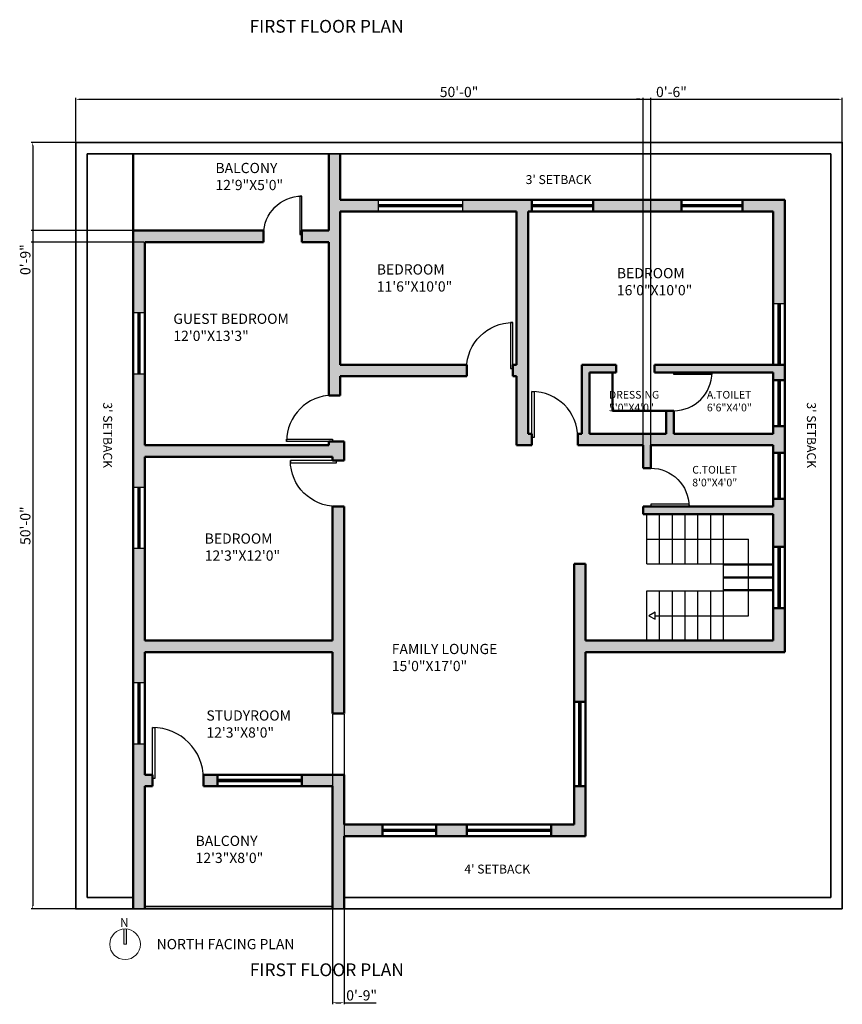
# Model space of a CAD drawing. Units: inches. Extents: x 2442 to 3851, y 589 to 2836.
# Tile 2 of 22: x 3165 to 3809, y 589 to 1359. Entities that reach past the tile are written whole.
import ezdxf

# ---------------------------------------------------------------- set-up
doc = ezdxf.new("R2010")
doc.units = ezdxf.units.IN
for name, color, linetype, lineweight in [('A-ANNO-DIMS', 2, 'Continuous', 18), ('A-ANNO-SYMB', 1, 'Continuous', 18), ('A-ANNO-TEXT', 7, 'Continuous', 18), ('A-AREA-IDEN', 7, 'Continuous', 18), ('A-DOOR', 4, 'Continuous', 25), ('A-FLOR-STRS', 3, 'Continuous', 25), ('A-GLAZ', 1, 'Continuous', 25), ('A-WALL', 7, 'Continuous', 50), ('A-WALL-PATT', 8, 'Continuous', 13), ('C-PROP', 7, 'Continuous', 35)]:
    doc.layers.add(name, color=color, linetype=linetype, lineweight=lineweight)
doc.styles.get("Standard").update_dxf_attribs({"font": 'arial.ttf'})
doc.dimstyles.new('ISO-25', dxfattribs={"dimtxt": 8, "dimasz": 2.5, "dimexe": 1.25, "dimexo": 0.625, "dimtad": 1, "dimlunit": 3, "dimtxsty": 'Standard', "dimcen": 2.5, "dimadec": 0, "dimazin": 0, "dimtfac": 1, "dimtmove": 0, "dimatfit": 3, "dimfxl": 1, "dimarcsym": 0})

# ---------------------------------------------------------------- blocks, each defined once
blk = doc.blocks.new('*U22')
for p, q in [((0, 0), (0, -6)), ((40, 0), (40, -6))]:
    blk.add_line(p, q)
blk.add_lwpolyline([(0, 0), (0, 40), (1.75, 40), (1.75, 0)], close=True)
blk.add_arc((0, 0), 40, 0, 90)
blk = doc.blocks.new('*U23')
for p, q in [((0, 0), (0, -6)), ((36, 0), (36, -6))]:
    blk.add_line(p, q)
blk.add_lwpolyline([(0, 0), (0, 36), (1.75, 36), (1.75, 0)], close=True)
blk.add_arc((0, 0), 36, 0, 90)
blk = doc.blocks.new('*U24')
for p, q in [((0, 0), (0, -6)), ((30, 0), (30, -6))]:
    blk.add_line(p, q)
blk.add_lwpolyline([(0, 0), (0, 30), (1.75, 30), (1.75, 0)], close=True)
blk.add_arc((0, 0), 30, 0, 90)
blk = doc.blocks.new('NORTH-ARROW')
at = {"transparency": 33554687}
h = blk.add_hatch(color=256, dxfattribs=at)
h.dxf.hatch_style = 1
h.paths.add_polyline_path([(13, 12), (11, 12), (11, 23.96, -0.020861), (12, 24, -0.020861), (13, 23.96)])
for p, q in [((11, 24), (11, 12)), ((13, 12), (13, 23.96)), ((11, 12), (13, 12))]:
    blk.add_line(p, q)
blk.add_circle((12, 12), 12)
blk.add_text('N', height=6.9).set_placement((7.98, 25.6))
blk = doc.blocks.new('*D261')
at = {"layer": 'A-ANNO-DIMS', "color": 0, "lineweight": -2, "transparency": 16777216}
for p, q in [((3209.02, 1263.95), (3209.02, 1298.32)), ((3211.52, 1297.07), (3806.52, 1297.07)), ((3809.02, 1263.95), (3809.02, 1298.32))]:
    blk.add_line(p, q, dxfattribs=at)
at = {"layer": 'A-ANNO-DIMS', "color": 0, "transparency": 16777216}
for points in [[(3211.52, 1297.49), (3211.52, 1296.66), (3209.02, 1297.07)], [(3806.52, 1297.49), (3806.52, 1296.66), (3809.02, 1297.07)]]:
    blk.add_solid(points, dxfattribs=at)
at = {"layer": 'Defpoints', "color": 0, "transparency": 16777216}
for p in [(3809.02, 1297.07), (3209.02, 1263.32), (3809.02, 1263.32)]:
    blk.add_point(p, dxfattribs=at)
at = {"layer": 'A-ANNO-DIMS', "color": 0, "transparency": 16777216, "insert": (3509.02, 1301.78), "char_height": 8, "attachment_point": 5}
blk.add_mtext('50\'-0"', dxfattribs=at)
blk = doc.blocks.new('*D262')
at = {"layer": 'A-ANNO-DIMS', "color": 0, "lineweight": -2, "transparency": 16777216}
for p, q in [((3208.4, 1263.32), (3174.02, 1263.32)), ((3175.27, 1260.82), (3175.27, 665.82)), ((3208.4, 663.32), (3174.02, 663.32))]:
    blk.add_line(p, q, dxfattribs=at)
at = {"layer": 'A-ANNO-DIMS', "color": 0, "transparency": 16777216}
for points in [[(3174.86, 1260.82), (3175.69, 1260.82), (3175.27, 1263.32)], [(3174.86, 665.82), (3175.69, 665.82), (3175.27, 663.32)]]:
    blk.add_solid(points, dxfattribs=at)
at = {"layer": 'Defpoints', "color": 0, "transparency": 16777216}
for p in [(3209.02, 1263.32), (3175.27, 663.32), (3209.02, 663.32)]:
    blk.add_point(p, dxfattribs=at)
at = {"layer": 'A-ANNO-DIMS', "color": 0, "transparency": 16777216, "insert": (3170.56, 963.32), "char_height": 8, "attachment_point": 5, "rotation": 90}
blk.add_mtext('50\'-0"', dxfattribs=at)
blk = doc.blocks.new('*D263')
at = {"layer": 'A-ANNO-DIMS', "color": 0, "lineweight": -2, "transparency": 16777216}
for p, q in [((3253.4, 1194.32), (3174.02, 1194.32)), ((3175.27, 1191.82), (3175.27, 1187.82)), ((3262.4, 1185.32), (3174.02, 1185.32)), ((3175.27, 1185.32), (3175.27, 1160.31))]:
    blk.add_line(p, q, dxfattribs=at)
at = {"layer": 'A-ANNO-DIMS', "color": 0, "transparency": 16777216}
for points in [[(3174.86, 1191.82), (3175.69, 1191.82), (3175.27, 1194.32)], [(3174.86, 1187.82), (3175.69, 1187.82), (3175.27, 1185.32)]]:
    blk.add_solid(points, dxfattribs=at)
at = {"layer": 'Defpoints', "color": 0, "transparency": 16777216}
for p in [(3254.02, 1194.32), (3175.27, 1185.32), (3263.02, 1185.32)]:
    blk.add_point(p, dxfattribs=at)
at = {"layer": 'A-ANNO-DIMS', "color": 0, "transparency": 16777216, "insert": (3170.56, 1171.56), "char_height": 8, "attachment_point": 5, "rotation": 90}
blk.add_mtext('0\'-9"', dxfattribs=at)
blk = doc.blocks.new('*D264')
at = {"layer": 'A-ANNO-DIMS', "color": 0, "lineweight": -2, "transparency": 16777216}
for p, q in [((3410.02, 815.7), (3410.02, 588.64)), ((3419.02, 815.7), (3419.02, 588.64)), ((3412.52, 589.89), (3416.52, 589.89)), ((3419.02, 589.89), (3444.04, 589.89))]:
    blk.add_line(p, q, dxfattribs=at)
at = {"layer": 'A-ANNO-DIMS', "color": 0, "transparency": 16777216}
for points in [[(3412.52, 590.31), (3412.52, 589.47), (3410.02, 589.89)], [(3416.52, 590.31), (3416.52, 589.47), (3419.02, 589.89)]]:
    blk.add_solid(points, dxfattribs=at)
at = {"layer": 'Defpoints', "color": 0, "transparency": 16777216}
for p in [(3410.02, 816.32), (3419.02, 816.32), (3419.02, 589.89)]:
    blk.add_point(p, dxfattribs=at)
at = {"layer": 'A-ANNO-DIMS', "color": 0, "transparency": 16777216, "insert": (3432.78, 594.6), "char_height": 8, "attachment_point": 5}
blk.add_mtext('0\'-9"', dxfattribs=at)
blk = doc.blocks.new('*D265')
at = {"layer": 'A-ANNO-DIMS', "color": 0, "lineweight": -2, "transparency": 16777216}
for p, q in [((3650.52, 1297.07), (3648.02, 1297.07)), ((3653.02, 1008.95), (3653.02, 1298.32)), ((3653.02, 1297.07), (3659.02, 1297.07)), ((3659.02, 1008.95), (3659.02, 1298.32)), ((3661.52, 1297.07), (3686.54, 1297.07))]:
    blk.add_line(p, q, dxfattribs=at)
at = {"layer": 'A-ANNO-DIMS', "color": 0, "transparency": 16777216}
for points in [[(3650.52, 1297.49), (3650.52, 1296.66), (3653.02, 1297.07)], [(3661.52, 1297.49), (3661.52, 1296.66), (3659.02, 1297.07)]]:
    blk.add_solid(points, dxfattribs=at)
at = {"layer": 'Defpoints', "color": 0, "transparency": 16777216}
for p in [(3659.02, 1297.07), (3653.02, 1008.32), (3659.02, 1008.32)]:
    blk.add_point(p, dxfattribs=at)
at = {"layer": 'A-ANNO-DIMS', "color": 0, "transparency": 16777216, "insert": (3675.28, 1301.78), "char_height": 8, "attachment_point": 5}
blk.add_mtext('0\'-6"', dxfattribs=at)

msp = doc.modelspace()

# ---------------------------------------------------------------- hatches: boundary and pattern name
at = {"layer": 'A-WALL-PATT'}
h = msp.add_hatch(color=256, dxfattribs=at)
h.dxf.hatch_style = 1
h.paths.add_polyline_path([(3356.024, 1185.323), (3356.024, 1191.323), (3356.024, 1194.323), (3254.024, 1194.323), (3254.024, 1129.823), (3263.024, 1129.823), (3263.024, 1185.323)])
h.paths.add_polyline_path([(3416.024, 1209.323), (3446.024, 1209.323), (3446.024, 1218.323), (3416.024, 1218.323), (3416.024, 1254.323), (3407.024, 1254.323), (3407.024, 1194.323), (3386.024, 1194.323), (3386.024, 1191.323), (3386.024, 1185.323), (3407.024, 1185.323), (3407.024, 1065.323), (3416.024, 1065.323), (3416.024, 1080.323), (3515.024, 1080.323), (3515.024, 1086.323), (3515.024, 1089.323), (3416.024, 1089.323)])
h.paths.add_polyline_path([(3563.024, 1209.323), (3566.024, 1209.323), (3566.024, 1218.323), (3512.024, 1218.323), (3512.024, 1209.323), (3554.024, 1209.323), (3554.024, 1089.323), (3551.024, 1089.323), (3551.024, 1086.323), (3551.024, 1080.323), (3554.024, 1080.323), (3554.024, 1026.323), (3566.024, 1026.323), (3566.024, 1032.323), (3566.024, 1035.323), (3563.024, 1035.323)])
h.paths.add_polyline_path([(3614.024, 1218.323), (3614.024, 1209.323), (3683.024, 1209.323), (3683.024, 1218.323)])
h.paths.add_polyline_path([(3755.024, 1209.323), (3755.024, 1137.323), (3764.024, 1137.323), (3764.024, 1218.323), (3731.024, 1218.323), (3731.024, 1209.323)])
h.paths.add_polyline_path([(3662.024, 1089.323), (3662.024, 1083.323), (3755.024, 1083.323), (3755.024, 1077.323), (3764.024, 1077.323), (3764.024, 1089.323)])
h.paths.add_polyline_path([(3755.024, 1026.323), (3755.024, 1020.323), (3764.024, 1020.323), (3764.024, 1041.323), (3755.024, 1041.323), (3755.024, 1035.323), (3677.024, 1035.323), (3677.024, 1053.323), (3671.024, 1053.323), (3671.024, 1035.323), (3611.024, 1035.323), (3611.024, 1083.323), (3632.024, 1083.323), (3632.024, 1089.323), (3605.024, 1089.323), (3605.024, 1035.323), (3602.024, 1035.323), (3602.024, 1026.323), (3653.024, 1026.323), (3653.024, 1008.323), (3659.024, 1008.323), (3659.024, 1026.323)])
h.paths.add_polyline_path([(3764.024, 984.323), (3755.024, 984.323), (3755.024, 978.323), (3653.024, 978.323), (3653.024, 972.323), (3755.024, 972.323), (3755.024, 946.823), (3764.024, 946.823)])
h.paths.add_polyline_path([(3608.024, 864.323), (3764.024, 864.323), (3764.024, 898.823), (3755.024, 898.823), (3755.024, 873.323), (3608.024, 873.323), (3608.024, 933.323), (3599.024, 933.323), (3599.024, 825.323), (3608.024, 825.323)])
h.paths.add_polyline_path([(3410.024, 873.323), (3263.024, 873.323), (3263.024, 945.323), (3254.024, 945.323), (3254.024, 840.323), (3263.024, 840.323), (3263.024, 864.323), (3410.024, 864.323), (3410.024, 816.323), (3419.024, 816.323), (3419.024, 978.323), (3413.024, 978.323), (3410.024, 978.323)])
h.paths.add_polyline_path([(3263.024, 1081.823), (3254.024, 1081.823), (3254.024, 993.323), (3263.024, 993.323), (3263.024, 1017.323), (3410.024, 1017.323), (3410.024, 1014.323), (3413.024, 1014.323), (3419.024, 1014.323), (3419.024, 1029.323), (3407.024, 1029.323), (3407.024, 1026.323), (3263.024, 1026.323)])
h.paths.add_polyline_path([(3254.024, 663.323), (3263.024, 663.323), (3263.024, 759.323), (3269.024, 759.323), (3269.024, 765.323), (3269.024, 768.323), (3263.024, 768.323), (3263.024, 792.323), (3254.024, 792.323)])
h.paths.add_polyline_path([(3419.024, 768.323), (3386.024, 768.323), (3386.024, 759.323), (3410.024, 759.323), (3410.024, 663.323), (3419.024, 663.323), (3419.024, 720.323), (3449.024, 720.323), (3449.024, 729.323), (3419.024, 729.323)])
h.paths.add_polyline_path([(3581.024, 720.323), (3608.024, 720.323), (3608.024, 759.323), (3599.024, 759.323), (3599.024, 729.323), (3581.024, 729.323)])
h.paths.add_polyline_path([(3491.024, 720.323), (3515.024, 720.323), (3515.024, 729.323), (3491.024, 729.323)])
h.paths.add_polyline_path([(3320.024, 768.323), (3309.024, 768.323), (3309.024, 759.323), (3320.024, 759.323)])
h.paths.add_polyline_path([(3282.007, 1103.379), (3387.059, 1103.379), (3387.059, 1133.793), (3282.007, 1133.793)], flags=9)
h.paths.add_polyline_path([(3511.253, 687.031), (3571.545, 687.031), (3571.545, 701.977), (3511.253, 701.977)], flags=9)
h.paths.add_polyline_path([(3777.335, 1062.03), (3777.335, 1001.738), (3792.281, 1001.738), (3792.281, 1062.03)], flags=9)
h.paths.add_polyline_path([(3558.97, 1226.744), (3619.262, 1226.744), (3619.262, 1241.69), (3558.97, 1241.69)], flags=9)
h.paths.add_polyline_path([(3314.979, 1221.433), (3377.263, 1221.433), (3377.263, 1251.848), (3314.979, 1251.848)], flags=9)
h.paths.add_polyline_path([(3624.453, 1049.367), (3671.045, 1049.367), (3671.045, 1072.178), (3624.453, 1072.178)], flags=25)
h.paths.add_polyline_path([(3701.15, 1049.367), (3744.07, 1049.367), (3744.07, 1072.178), (3701.15, 1072.178)], flags=25)
h.paths.add_polyline_path([(3689.533, 990.66), (3731.868, 990.66), (3731.868, 1013.471), (3689.533, 1013.471)], flags=9)
h.paths.add_polyline_path([(3629.196, 1139.095), (3693.452, 1139.095), (3693.452, 1169.509), (3629.196, 1169.509)], flags=9)
h.paths.add_polyline_path([(3441.284, 1142.006), (3505.54, 1142.006), (3505.54, 1172.421), (3441.284, 1172.421)], flags=25)
h.paths.add_polyline_path([(3306.565, 931.348), (3370.821, 931.348), (3370.821, 961.763), (3306.565, 961.763)], flags=25)
h.paths.add_polyline_path([(3307.889, 792.848), (3387.355, 792.848), (3387.355, 823.263), (3307.889, 823.263)], flags=9)
h.paths.add_polyline_path([(3452.987, 844.909), (3554.971, 844.909), (3554.971, 875.324), (3452.987, 875.324)], flags=9)

# ---------------------------------------------------------------- linework, layer by layer
at = {"layer": 'A-FLOR-STRS'}
for p, q in [((3656.024, 933.323), (3656.024, 972.323)), ((3666.024, 933.323), (3666.024, 972.323)), ((3676.024, 933.323), (3676.024, 972.323)), ((3686.024, 933.323), (3686.024, 972.323)), ((3696.024, 933.323), (3696.024, 972.323)), ((3706.024, 933.323), (3706.024, 972.323)), ((3716.024, 912.323), (3716.024, 972.323)), ((3656.024, 952.823), (3735.524, 952.823)), ((3735.524, 892.823), (3735.524, 952.823)), ((3656.024, 933.323), (3716.024, 933.323)), ((3656.024, 912.323), (3716.024, 912.323)), ((3662.482, 892.823), (3735.524, 892.823))]:
    msp.add_line(p, q, dxfattribs=at)
at = {"layer": 'A-FLOR-STRS', "ltscale": 0.5}
for p, q in [((3656.024, 873.323), (3656.024, 912.323)), ((3666.024, 873.323), (3666.024, 912.323)), ((3676.024, 873.323), (3676.024, 912.323)), ((3686.024, 873.323), (3686.024, 912.323)), ((3696.024, 873.323), (3696.024, 912.323)), ((3706.024, 873.323), (3706.024, 912.323)), ((3716.024, 873.323), (3716.024, 912.323))]:
    msp.add_line(p, q, dxfattribs=at)
at = {"layer": 'A-FLOR-STRS'}
msp.add_lwpolyline([(3657.639, 892.823), (3662.482, 890.027), (3662.482, 895.619)], close=True, dxfattribs=at)
at = {"layer": 'A-GLAZ'}
for p, q in [((3446.024, 1209.323), (3446.024, 1218.323)), ((3512.024, 1209.323), (3512.024, 1218.323)), ((3755.024, 1137.323), (3764.024, 1137.323)), ((3263.024, 1129.823), (3254.024, 1129.823)), ((3263.024, 1081.823), (3254.024, 1081.823)), ((3263.024, 993.323), (3254.024, 993.323)), ((3263.024, 945.323), (3254.024, 945.323)), ((3263.024, 840.323), (3254.024, 840.323)), ((3263.024, 792.323), (3254.024, 792.323))]:
    msp.add_line(p, q, dxfattribs=at)
at = {"layer": 'A-WALL'}
for p, q in [((3254.024, 1254.323), (3254.024, 663.323)), ((3407.024, 1194.323), (3407.024, 1254.323)), ((3416.024, 1218.323), (3416.024, 1254.323)), ((3416.024, 1218.323), (3764.024, 1218.323)), ((3566.024, 1209.323), (3566.024, 1218.323)), ((3614.024, 1209.323), (3614.024, 1218.323)), ((3683.024, 1209.323), (3683.024, 1218.323)), ((3731.024, 1209.323), (3731.024, 1218.323)), ((3764.024, 864.323), (3764.024, 1218.323)), ((3446.024, 1214.323), (3512.024, 1214.323)), ((3446.024, 1213.323), (3512.024, 1213.323)), ((3566.024, 1214.323), (3614.024, 1214.323)), ((3566.024, 1213.323), (3614.024, 1213.323)), ((3683.024, 1214.323), (3731.024, 1214.323)), ((3683.024, 1213.323), (3731.024, 1213.323)), ((3416.024, 1089.323), (3416.024, 1209.323)), ((3416.024, 1209.323), (3554.024, 1209.323)), ((3554.024, 1089.323), (3554.024, 1209.323)), ((3563.024, 1035.323), (3563.024, 1209.323)), ((3563.024, 1209.323), (3755.024, 1209.323)), ((3755.024, 1089.323), (3755.024, 1209.323)), ((3254.024, 1194.323), (3356.024, 1194.323)), ((3356.024, 1185.323), (3356.024, 1194.323)), ((3386.024, 1185.323), (3386.024, 1194.323)), ((3386.024, 1194.323), (3407.024, 1194.323)), ((3263.024, 1185.323), (3263.024, 1026.323)), ((3263.024, 1185.323), (3356.024, 1185.323)), ((3386.024, 1185.323), (3407.024, 1185.323)), ((3407.024, 1065.323), (3407.024, 1185.323)), ((3759.024, 1089.323), (3759.024, 1137.323)), ((3760.024, 1089.323), (3760.024, 1137.323)), ((3258.024, 1129.823), (3258.024, 1081.823)), ((3259.024, 1129.823), (3259.024, 1081.823)), ((3416.024, 1089.323), (3515.024, 1089.323)), ((3515.024, 1080.323), (3515.024, 1089.323)), ((3551.024, 1080.323), (3551.024, 1089.323)), ((3551.024, 1089.323), (3554.024, 1089.323)), ((3605.024, 1035.323), (3605.024, 1089.323)), ((3605.024, 1089.323), (3632.024, 1089.323)), ((3632.024, 1083.323), (3632.024, 1089.323)), ((3662.024, 1083.323), (3662.024, 1089.323)), ((3662.024, 1089.323), (3764.024, 1089.323)), ((3416.024, 1065.323), (3416.024, 1080.323)), ((3416.024, 1080.323), (3515.024, 1080.323)), ((3551.024, 1080.323), (3554.024, 1080.323)), ((3554.024, 1026.323), (3554.024, 1080.323)), ((3611.024, 1035.323), (3611.024, 1083.323)), ((3611.024, 1083.323), (3632.024, 1083.323)), ((3629.024, 1053.323), (3629.024, 1083.323)), ((3662.024, 1083.323), (3755.024, 1083.323)), ((3755.024, 1035.323), (3755.024, 1083.323)), ((3755.024, 1077.323), (3764.024, 1077.323)), ((3759.024, 1041.323), (3759.024, 1077.323)), ((3760.024, 1041.323), (3760.024, 1077.323)), ((3407.024, 1065.323), (3416.024, 1065.323)), ((3629.024, 1053.323), (3671.024, 1053.323)), ((3671.024, 1035.323), (3671.024, 1053.323)), ((3671.024, 1053.323), (3677.024, 1053.323)), ((3677.024, 1035.323), (3677.024, 1053.323)), ((3755.024, 1041.323), (3764.024, 1041.323)), ((3563.024, 1035.323), (3566.024, 1035.323)), ((3566.024, 1026.323), (3566.024, 1035.323)), ((3602.024, 1026.323), (3602.024, 1035.323)), ((3602.024, 1035.323), (3605.024, 1035.323)), ((3611.024, 1035.323), (3671.024, 1035.323)), ((3677.024, 1035.323), (3755.024, 1035.323)), ((3263.024, 1026.323), (3407.024, 1026.323)), ((3407.024, 1026.323), (3407.024, 1029.323)), ((3407.024, 1029.323), (3419.024, 1029.323)), ((3419.024, 1014.323), (3419.024, 1029.323)), ((3554.024, 1026.323), (3566.024, 1026.323)), ((3602.024, 1026.323), (3653.024, 1026.323)), ((3653.024, 1008.323), (3653.024, 1026.323)), ((3659.024, 1008.323), (3659.024, 1026.323)), ((3659.024, 1026.323), (3755.024, 1026.323)), ((3755.024, 978.323), (3755.024, 1026.323)), ((3755.024, 1020.323), (3764.024, 1020.323)), ((3759.024, 984.323), (3759.024, 1020.323)), ((3760.024, 984.323), (3760.024, 1020.323)), ((3263.024, 1017.323), (3263.024, 873.323)), ((3263.024, 1017.323), (3410.024, 1017.323)), ((3410.024, 1014.323), (3410.024, 1017.323)), ((3410.024, 1014.323), (3419.024, 1014.323)), ((3653.024, 1008.323), (3659.024, 1008.323)), ((3258.024, 993.323), (3258.024, 945.323)), ((3259.024, 993.323), (3259.024, 945.323)), ((3755.024, 984.323), (3764.024, 984.323)), ((3410.024, 873.323), (3410.024, 978.323)), ((3410.024, 978.323), (3419.024, 978.323)), ((3419.024, 816.323), (3419.024, 978.323)), ((3653.024, 972.323), (3653.024, 978.323)), ((3653.024, 978.323), (3755.024, 978.323)), ((3653.024, 972.323), (3755.024, 972.323)), ((3755.024, 873.323), (3755.024, 972.323)), ((3755.024, 946.823), (3764.024, 946.823)), ((3759.024, 898.823), (3759.024, 946.823)), ((3760.024, 898.823), (3760.024, 946.823)), ((3599.024, 933.323), (3608.024, 933.323)), ((3599.024, 729.323), (3599.024, 933.323)), ((3608.024, 873.323), (3608.024, 933.323)), ((3716.024, 932.823), (3755.024, 932.823)), ((3716.024, 922.823), (3755.024, 922.823)), ((3716.024, 912.823), (3755.024, 912.823)), ((3755.024, 898.823), (3764.024, 898.823)), ((3263.024, 873.323), (3410.024, 873.323)), ((3608.024, 873.323), (3755.024, 873.323)), ((3263.024, 864.323), (3263.024, 768.323)), ((3263.024, 864.323), (3410.024, 864.323)), ((3410.024, 816.323), (3410.024, 864.323)), ((3608.024, 720.323), (3608.024, 864.323)), ((3608.024, 864.323), (3764.024, 864.323)), ((3258.024, 840.323), (3258.024, 792.323)), ((3259.024, 840.323), (3259.024, 792.323)), ((3599.024, 825.323), (3608.024, 825.323)), ((3603.024, 759.323), (3603.024, 825.323)), ((3604.024, 759.323), (3604.024, 825.323)), ((3410.024, 816.323), (3419.024, 816.323)), ((3263.024, 768.323), (3269.024, 768.323)), ((3269.024, 768.323), (3269.024, 759.323)), ((3309.024, 768.323), (3309.024, 759.323)), ((3309.024, 768.323), (3419.024, 768.323)), ((3320.024, 759.323), (3320.024, 768.323)), ((3320.024, 764.323), (3386.024, 764.323)), ((3320.024, 763.323), (3386.024, 763.323)), ((3386.024, 759.323), (3386.024, 768.323)), ((3419.024, 729.323), (3419.024, 768.323)), ((3263.024, 759.323), (3263.024, 663.323)), ((3263.024, 759.323), (3269.024, 759.323)), ((3309.024, 759.323), (3410.024, 759.323)), ((3410.024, 663.323), (3410.024, 759.323)), ((3599.024, 759.323), (3608.024, 759.323)), ((3419.024, 729.323), (3599.024, 729.323)), ((3449.024, 720.323), (3449.024, 729.323)), ((3449.024, 725.323), (3491.024, 725.323)), ((3491.024, 720.323), (3491.024, 729.323)), ((3515.024, 720.323), (3515.024, 729.323)), ((3515.024, 725.323), (3581.024, 725.323)), ((3581.024, 720.323), (3581.024, 729.323)), ((3419.024, 720.323), (3608.024, 720.323)), ((3419.024, 663.323), (3419.024, 720.323)), ((3449.024, 724.323), (3491.024, 724.323)), ((3515.024, 724.323), (3581.024, 724.323))]:
    msp.add_line(p, q, dxfattribs=at)
at = {"layer": 'C-PROP'}
for points in [[(3809.024, 663.323), (3809.024, 1263.323), (3209.024, 1263.323), (3209.024, 663.323), (3809.024, 663.323)], [(3800.024, 672.323), (3800.024, 1254.323), (3218.024, 1254.323), (3218.024, 672.323), (3254.024, 672.323)], [(3419.024, 672.323), (3800.024, 672.323)], [(3263.024, 665.323), (3410.024, 665.323)]]:
    msp.add_lwpolyline(points, dxfattribs=at)

# ---------------------------------------------------------------- block references
at = {"layer": 'A-ANNO-SYMB'}
msp.add_blockref('NORTH-ARROW', (3235.614, 623.64), dxfattribs=at)
at = {"layer": 'A-DOOR', "xscale": -1}
for name, p in [('*U24', (3386.024, 1191.323)), ('*U23', (3551.024, 1086.323))]:
    msp.add_blockref(name, p, dxfattribs=at)
at = {"layer": 'A-DOOR'}
for name, p, rotation in [('*U24', (3677.024, 1083.323), 269.9999999999969), ('*U23', (3410.024, 1029.323), 90.00000000000003)]:
    msp.add_blockref(name, p, dxfattribs=dict(at, rotation=rotation))
for name, p in [('*U23', (3566.024, 1032.323)), ('*U22', (3269.024, 765.323))]:
    msp.add_blockref(name, p, dxfattribs=at)
at = {"layer": 'A-DOOR', "xscale": -1}
for name, p, rotation in [('*U23', (3413.024, 1014.323), 90), ('*U24', (3659.024, 978.323), 270)]:
    msp.add_blockref(name, p, dxfattribs=dict(at, rotation=rotation))

# ---------------------------------------------------------------- texts
at = {"layer": 'A-ANNO-TEXT', "attachment_point": 1}
for s, width, insert, char_height in [('{\\fTimes New Roman|b0|i0|c0|p18;FIRST FLOOR PLAN}', 196.26071, (3344.992, 1359.217), 10), ("{\\fTimes New Roman|b0|i0|c0|p18;3' SETBACK}", 79.56037, (3561.139, 1237.73), 7), ("{\\fTimes New Roman|b0|i0|c0|p18;4' SETBACK}", 79.56037, (3513.164, 698.017), 7), ('{\\fTimes New Roman|b0|i0|c0|p18;NORTH FACING PLAN}', 196.26071, (3272.307, 639.763), 8), ('{\\fTimes New Roman|b0|i0|c0|p18;FIRST FLOOR PLAN}', 196.26071, (3345.219, 620.676), 10)]:
    msp.add_mtext_dynamic_manual_height_columns(s, width=width, gutter_width=12.5, heights=[0], dxfattribs=dict(at, insert=insert, char_height=char_height))
at = {"layer": 'A-ANNO-TEXT', "char_height": 7, "attachment_point": 1, "rotation": 270}
for insert in [(3237.481, 1059.862), (3788.321, 1059.862)]:
    msp.add_mtext_dynamic_manual_height_columns("{\\fTimes New Roman|b0|i0|c0|p18;3' SETBACK}", width=79.56037, gutter_width=12.5, heights=[0], dxfattribs=dict(at, insert=insert))
at = {"layer": 'A-AREA-IDEN', "attachment_point": 1}
for s, insert, char_height in [('{\\fTimes New Roman|b0|i0|c0|p18;BALCONY\\P12\'9"X5\'0"}', (3318.363, 1247.321), 8), ('{\\fTimes New Roman|b0|i0|c0|p18;BEDROOM\\P11\'6"X10\'0"}', (3444.668, 1167.895), 8), ('{\\fTimes New Roman|b0|i0|c0|p18;BEDROOM\\P16\'0"X10\'0"}', (3632.58, 1164.983), 8), ('{\\fTimes New Roman|b0|i0|c0|p18;GUEST BEDROOM\\P12\'0"X13\'3"}', (3285.391, 1129.267), 8), ('{\\fTimes New Roman|b0|i0|c0|p18;DRESSING\\P5\'0"X4\'0"}', (3626.377, 1068.783), 6), ('{\\fTimes New Roman|b0|i0|c0|p18;A.TOILET\\P6\'6"X4\'0"}', (3703.031, 1068.783), 6), ('{\\fTimes New Roman|b0|i0|c0|p18;C.TOILET\\P8\'0"X4\'0"}', (3691.569, 1010.077), 6), ('{\\fTimes New Roman|b0|i0|c0|p18;BEDROOM\\P12\'3"X12\'0"}', (3309.949, 957.237), 8), ('{\\fTimes New Roman|b0|i0|c0|p18;FAMILY LOUNGE\\P15\'0"X17\'0"}', (3456.372, 870.797), 8), ('{\\fTimes New Roman|b0|i0|c0|p18;STUDYROOM\\P12\'3"X8\'0"}', (3311.273, 818.736), 8), ('{\\fTimes New Roman|b0|i0|c0|p18;BALCONY\\P12\'3"X8\'0"}', (3302.804, 720.58), 8)]:
    msp.add_mtext_dynamic_manual_height_columns(s, width=110.76054, gutter_width=12.5, heights=[0], dxfattribs=dict(at, insert=insert, char_height=char_height))

# ---------------------------------------------------------------- dimensions: what is measured, and where the dimension line sits
at = {"layer": 'A-ANNO-DIMS'}
for base, p1, p2, picture, middle in [((3809.024, 1297.073), (3209.024, 1263.323), (3809.024, 1263.323), '*D261', (3509.024, 1301.782)), ((3659.024, 1297.073), (3653.024, 1008.323), (3659.024, 1008.323), '*D265', (3675.283, 1301.782)), ((3419.024, 589.89), (3410.024, 816.323), (3419.024, 816.323), '*D264', (3432.783, 594.6))]:
    dim = msp.add_linear_dim(base=base, p1=p1, p2=p2, dimstyle='ISO-25', override={"dimdec": 1, "dimlfac": 1, "dimrnd": 0, "dimzin": 1, "dimdsep": 46, "dimlunit": 4, "dimfrac": 2}, dxfattribs=at)
    dim.commit()
    dim.dimension.update_dxf_attribs({"geometry": picture, "text_midpoint": middle})
for base, p1, p2, picture, middle in [((3175.274, 663.323), (3209.024, 1263.323), (3209.024, 663.323), '*D262', (3170.565, 963.323)), ((3175.274, 1185.323), (3254.024, 1194.323), (3263.024, 1185.323), '*D263', (3170.565, 1171.565))]:
    dim = msp.add_linear_dim(base=base, p1=p1, p2=p2, angle=90, dimstyle='ISO-25', override={"dimdec": 1, "dimlfac": 1, "dimrnd": 0, "dimzin": 1, "dimdsep": 46, "dimlunit": 4, "dimfrac": 2}, dxfattribs=at)
    dim.commit()
    dim.dimension.update_dxf_attribs({"geometry": picture, "text_midpoint": middle})

doc.saveas('drawing.dxf')
